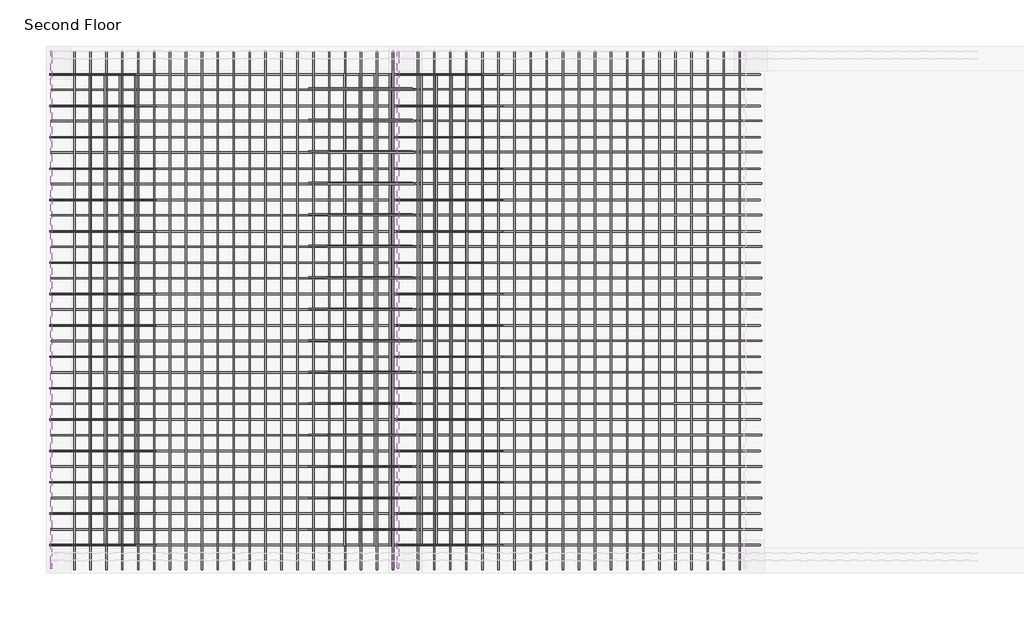
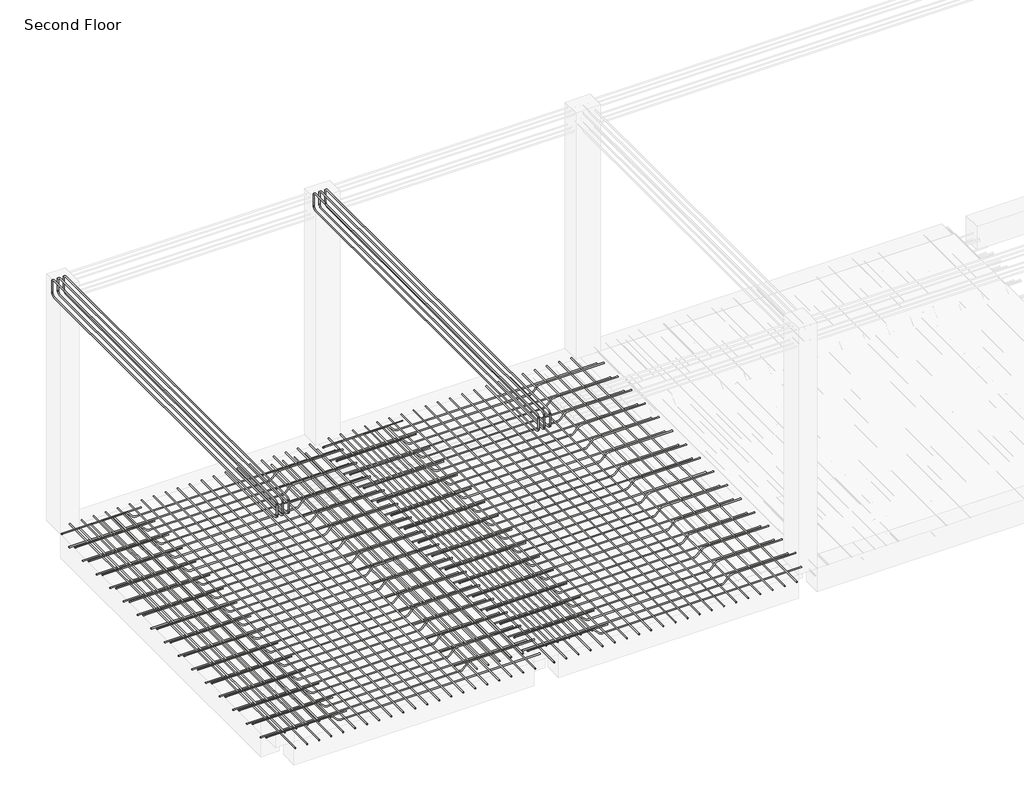
# One storey, part 2 of 4: 16 reinforcing bars.
"""IFC4 building model written with IfcOpenShell, lengths in millimetres."""

from ifc_helpers import new_model, si_unit, point, frame, origin, place, context, project, spatial, polyline, circle_curve, trimmed, segment, composite_curve, source, transform, mapped, element, save
from ifc_brep_helpers import swept_disk

model = new_model("IFC4")

# Units and contexts
model_context = context("Model", 3, world=origin())
ifc_project = project(units=[si_unit("LENGTHUNIT", "METRE", prefix="MILLI")], contexts=[model_context])

# Site, building, storey
site = spatial("IfcSite", under=ifc_project)
building = spatial("IfcBuilding", under=site)
storey = spatial("IfcBuildingStorey", under=building, Name="Second Floor", Elevation=6400.8)

# Reinforcing bars
placement = place(None, origin())
reinforcing_bar_shape = source(origin(), model_context, "Body", "SolidModel", [
    swept_disk(composite_curve([segment(polyline([(-6122.7112474, 5017.2334631, 9364.0994949), (-6122.7112474, 5017.2334631, 9512.0994949)]), True, "CONTINUOUS"), segment(trimmed(circle_curve(frame((-6122.7112474, 4971.2334631, 9512.0994949), z_axis=(1.0, 0.0, 0.0), x_axis=(0.0, 46.0, 0.0)), 46.0), [point((-6122.7112474, 5017.2334631, 9512.0994949))], [point((-6122.7112474, 4971.2334631, 9558.0994949))], True, "CARTESIAN"), True, "CONTINUOUS"), segment(polyline([(-6122.7112474, 4971.2334631, 9558.0994949), (-6122.7112474, 278.4334631, 9558.0994949)]), True, "CONTINUOUS"), segment(trimmed(circle_curve(frame((-6122.7112474, 278.4334631, 9512.0994949), z_axis=(1.0, 0.0, 0.0), x_axis=(0.0, 0.0, 46.0)), 46.0), [point((-6122.7112474, 278.4334631, 9558.0994949))], [point((-6122.7112474, 232.4334631, 9512.0994949))], True, "CARTESIAN"), True, "CONTINUOUS"), segment(polyline([(-6122.7112474, 232.4334631, 9512.0994949), (-6122.7112474, 232.4334631, 9364.0994949)]), True, "CONTINUOUS")], self_intersect=False), 6.0),
])
element("IfcReinforcingBar", 1, at=placement, inside=storey, context=model_context, shape_type="MappedRepresentation", body=[
    mapped(reinforcing_bar_shape, transform((0.0, 0.0, 0.0), x_axis=(1.0, 0.0, 0.0), y_axis=(0.0, 1.0, 0.0), z_axis=(0.0, 0.0, 1.0))),
    mapped(reinforcing_bar_shape, transform((71.1994949, 0.0, 0.0), x_axis=(1.0, 0.0, 0.0), y_axis=(0.0, 1.0, 0.0), z_axis=(0.0, 0.0, 1.0))),
    mapped(reinforcing_bar_shape, transform((142.3989899, 0.0, 0.0), x_axis=(1.0, 0.0, 0.0), y_axis=(0.0, 1.0, 0.0), z_axis=(0.0, 0.0, 1.0))),
])
reinforcing_bar_2_shape = source(origin(), model_context, "Body", "SolidModel", [
    swept_disk(composite_curve([segment(polyline([(-6122.7112474, 5017.2334631, 9533.5005051), (-6122.7112474, 5017.2334631, 9385.5005051)]), True, "CONTINUOUS"), segment(trimmed(circle_curve(frame((-6122.7112474, 4971.2334631, 9385.5005051), z_axis=(-1.0, 0.0, 0.0), x_axis=(0.0, 46.0, 0.0)), 46.0), [point((-6122.7112474, 5017.2334631, 9385.5005051))], [point((-6122.7112474, 4971.2334631, 9339.5005051))], True, "CARTESIAN"), True, "CONTINUOUS"), segment(polyline([(-6122.7112474, 4971.2334631, 9339.5005051), (-6122.7112474, 278.4334631, 9339.5005051)]), True, "CONTINUOUS"), segment(trimmed(circle_curve(frame((-6122.7112474, 278.4334631, 9385.5005051), z_axis=(-1.0, 0.0, 0.0), x_axis=(0.0, 0.0, -46.0)), 46.0), [point((-6122.7112474, 278.4334631, 9339.5005051))], [point((-6122.7112474, 232.4334631, 9385.5005051))], True, "CARTESIAN"), True, "CONTINUOUS"), segment(polyline([(-6122.7112474, 232.4334631, 9385.5005051), (-6122.7112474, 232.4334631, 9533.5005051)]), True, "CONTINUOUS")], self_intersect=False), 6.0),
])
element("IfcReinforcingBar", 2, at=placement, inside=storey, context=model_context, shape_type="MappedRepresentation", body=[
    mapped(reinforcing_bar_2_shape, transform((0.0, 0.0, 0.0), x_axis=(1.0, 0.0, 0.0), y_axis=(0.0, 1.0, 0.0), z_axis=(0.0, 0.0, 1.0))),
    mapped(reinforcing_bar_2_shape, transform((71.1994949, 0.0, 0.0), x_axis=(1.0, 0.0, 0.0), y_axis=(0.0, 1.0, 0.0), z_axis=(0.0, 0.0, 1.0))),
    mapped(reinforcing_bar_2_shape, transform((142.3989899, 0.0, 0.0), x_axis=(1.0, 0.0, 0.0), y_axis=(0.0, 1.0, 0.0), z_axis=(0.0, 0.0, 1.0))),
])
reinforcing_bar_3_shape = source(origin(), model_context, "Body", "SolidModel", [
    swept_disk(composite_curve([segment(polyline([(-9335.8112474, 5017.2334631, 9364.0994949), (-9335.8112474, 5017.2334631, 9512.0994949)]), True, "CONTINUOUS"), segment(trimmed(circle_curve(frame((-9335.8112474, 4971.2334631, 9512.0994949), z_axis=(1.0, 0.0, 0.0), x_axis=(0.0, 46.0, 0.0)), 46.0), [point((-9335.8112474, 5017.2334631, 9512.0994949))], [point((-9335.8112474, 4971.2334631, 9558.0994949))], True, "CARTESIAN"), True, "CONTINUOUS"), segment(polyline([(-9335.8112474, 4971.2334631, 9558.0994949), (-9335.8112474, 278.4334631, 9558.0994949)]), True, "CONTINUOUS"), segment(trimmed(circle_curve(frame((-9335.8112474, 278.4334631, 9512.0994949), z_axis=(1.0, 0.0, 0.0), x_axis=(0.0, 0.0, 46.0)), 46.0), [point((-9335.8112474, 278.4334631, 9558.0994949))], [point((-9335.8112474, 232.4334631, 9512.0994949))], True, "CARTESIAN"), True, "CONTINUOUS"), segment(polyline([(-9335.8112474, 232.4334631, 9512.0994949), (-9335.8112474, 232.4334631, 9364.0994949)]), True, "CONTINUOUS")], self_intersect=False), 6.0),
])
element("IfcReinforcingBar", 3, at=placement, inside=storey, context=model_context, shape_type="MappedRepresentation", body=[
    mapped(reinforcing_bar_3_shape, transform((0.0, 0.0, 0.0), x_axis=(1.0, 0.0, 0.0), y_axis=(0.0, 1.0, 0.0), z_axis=(0.0, 0.0, 1.0))),
    mapped(reinforcing_bar_3_shape, transform((71.1994949, 0.0, 0.0), x_axis=(1.0, 0.0, 0.0), y_axis=(0.0, 1.0, 0.0), z_axis=(0.0, 0.0, 1.0))),
    mapped(reinforcing_bar_3_shape, transform((142.3989899, 0.0, 0.0), x_axis=(1.0, 0.0, 0.0), y_axis=(0.0, 1.0, 0.0), z_axis=(0.0, 0.0, 1.0))),
])
reinforcing_bar_4_shape = source(origin(), model_context, "Body", "SolidModel", [
    swept_disk(composite_curve([segment(polyline([(-9335.8112474, 5017.2334631, 9533.5005051), (-9335.8112474, 5017.2334631, 9385.5005051)]), True, "CONTINUOUS"), segment(trimmed(circle_curve(frame((-9335.8112474, 4971.2334631, 9385.5005051), z_axis=(-1.0, 0.0, 0.0), x_axis=(0.0, 46.0, 0.0)), 46.0), [point((-9335.8112474, 5017.2334631, 9385.5005051))], [point((-9335.8112474, 4971.2334631, 9339.5005051))], True, "CARTESIAN"), True, "CONTINUOUS"), segment(polyline([(-9335.8112474, 4971.2334631, 9339.5005051), (-9335.8112474, 278.4334631, 9339.5005051)]), True, "CONTINUOUS"), segment(trimmed(circle_curve(frame((-9335.8112474, 278.4334631, 9385.5005051), z_axis=(-1.0, 0.0, 0.0), x_axis=(0.0, 0.0, -46.0)), 46.0), [point((-9335.8112474, 278.4334631, 9339.5005051))], [point((-9335.8112474, 232.4334631, 9385.5005051))], True, "CARTESIAN"), True, "CONTINUOUS"), segment(polyline([(-9335.8112474, 232.4334631, 9385.5005051), (-9335.8112474, 232.4334631, 9533.5005051)]), True, "CONTINUOUS")], self_intersect=False), 6.0),
])
element("IfcReinforcingBar", 4, at=placement, inside=storey, context=model_context, shape_type="MappedRepresentation", body=[
    mapped(reinforcing_bar_4_shape, transform((0.0, 0.0, 0.0), x_axis=(1.0, 0.0, 0.0), y_axis=(0.0, 1.0, 0.0), z_axis=(0.0, 0.0, 1.0))),
    mapped(reinforcing_bar_4_shape, transform((71.1994949, 0.0, 0.0), x_axis=(1.0, 0.0, 0.0), y_axis=(0.0, 1.0, 0.0), z_axis=(0.0, 0.0, 1.0))),
    mapped(reinforcing_bar_4_shape, transform((142.3989899, 0.0, 0.0), x_axis=(1.0, 0.0, 0.0), y_axis=(0.0, 1.0, 0.0), z_axis=(0.0, 0.0, 1.0))),
])
reinforcing_bar_5_shape = source(origin(), model_context, "Body", "SolidModel", [
    swept_disk(composite_curve([segment(polyline([(-9347.5125695, 4803.6334631, 6369.8), (-8565.5792829, 4803.6334631, 6369.8)]), True, "CONTINUOUS"), segment(trimmed(circle_curve(frame((-8565.5792829, 4803.6334631, 6323.8), z_axis=(0.0, 1.0, 0.0), x_axis=(0.0, 0.0, 46.0)), 46.0), [point((-8565.5792829, 4803.6334631, 6369.8))], [point((-8533.052371, 4803.6334631, 6356.3269119))], True, "CARTESIAN"), True, "CONTINUOUS"), segment(polyline([(-8533.052371, 4803.6334631, 6356.3269119), (-8469.5985471, 4803.6334631, 6292.8730881)]), True, "CONTINUOUS"), segment(trimmed(circle_curve(frame((-8437.0716352, 4803.6334631, 6325.4), z_axis=(0.0, -1.0000000000000002, 0.0), x_axis=(-32.526911900000414, 0.0, -32.526911899999504)), 46.0), [point((-8469.5985471, 4803.6334631, 6292.8730881))], [point((-8437.0716352, 4803.6334631, 6279.4))], True, "CARTESIAN"), True, "CONTINUOUS"), segment(polyline([(-8437.0716352, 4803.6334631, 6279.4), (-5982.0597449, 4803.6334631, 6279.4)]), True, "CONTINUOUS")], self_intersect=False), 6.0),
])
element("IfcReinforcingBar", 5, at=placement, inside=storey, context=model_context, shape_type="MappedRepresentation", body=[
    mapped(reinforcing_bar_5_shape, transform((0.0, 0.0, 0.0), x_axis=(1.0, 0.0, 0.0), y_axis=(0.0, 1.0, 0.0), z_axis=(0.0, 0.0, 1.0))),
    mapped(reinforcing_bar_5_shape, transform((0.0, -290.5066667, 0.0), x_axis=(1.0, 0.0, 0.0), y_axis=(0.0, 1.0, 0.0), z_axis=(0.0, 0.0, 1.0))),
    mapped(reinforcing_bar_5_shape, transform((0.0, -581.0133333, 0.0), x_axis=(1.0, 0.0, 0.0), y_axis=(0.0, 1.0, 0.0), z_axis=(0.0, 0.0, 1.0))),
    mapped(reinforcing_bar_5_shape, transform((0.0, -871.52, 0.0), x_axis=(1.0, 0.0, 0.0), y_axis=(0.0, 1.0, 0.0), z_axis=(0.0, 0.0, 1.0))),
    mapped(reinforcing_bar_5_shape, transform((0.0, -1162.0266667, 0.0), x_axis=(1.0, 0.0, 0.0), y_axis=(0.0, 1.0, 0.0), z_axis=(0.0, 0.0, 1.0))),
    mapped(reinforcing_bar_5_shape, transform((0.0, -1452.5333333, 0.0), x_axis=(1.0, 0.0, 0.0), y_axis=(0.0, 1.0, 0.0), z_axis=(0.0, 0.0, 1.0))),
    mapped(reinforcing_bar_5_shape, transform((0.0, -1743.04, 0.0), x_axis=(1.0, 0.0, 0.0), y_axis=(0.0, 1.0, 0.0), z_axis=(0.0, 0.0, 1.0))),
    mapped(reinforcing_bar_5_shape, transform((0.0, -2033.5466667, 0.0), x_axis=(1.0, 0.0, 0.0), y_axis=(0.0, 1.0, 0.0), z_axis=(0.0, 0.0, 1.0))),
    mapped(reinforcing_bar_5_shape, transform((0.0, -2324.0533333, 0.0), x_axis=(1.0, 0.0, 0.0), y_axis=(0.0, 1.0, 0.0), z_axis=(0.0, 0.0, 1.0))),
    mapped(reinforcing_bar_5_shape, transform((0.0, -2614.56, 0.0), x_axis=(1.0, 0.0, 0.0), y_axis=(0.0, 1.0, 0.0), z_axis=(0.0, 0.0, 1.0))),
    mapped(reinforcing_bar_5_shape, transform((0.0, -2905.0666667, 0.0), x_axis=(1.0, 0.0, 0.0), y_axis=(0.0, 1.0, 0.0), z_axis=(0.0, 0.0, 1.0))),
    mapped(reinforcing_bar_5_shape, transform((0.0, -3195.5733333, 0.0), x_axis=(1.0, 0.0, 0.0), y_axis=(0.0, 1.0, 0.0), z_axis=(0.0, 0.0, 1.0))),
    mapped(reinforcing_bar_5_shape, transform((0.0, -3486.08, 0.0), x_axis=(1.0, 0.0, 0.0), y_axis=(0.0, 1.0, 0.0), z_axis=(0.0, 0.0, 1.0))),
    mapped(reinforcing_bar_5_shape, transform((0.0, -3776.5866667, 0.0), x_axis=(1.0, 0.0, 0.0), y_axis=(0.0, 1.0, 0.0), z_axis=(0.0, 0.0, 1.0))),
    mapped(reinforcing_bar_5_shape, transform((0.0, -4067.0933333, 0.0), x_axis=(1.0, 0.0, 0.0), y_axis=(0.0, 1.0, 0.0), z_axis=(0.0, 0.0, 1.0))),
    mapped(reinforcing_bar_5_shape, transform((0.0, -4357.6, 0.0), x_axis=(1.0, 0.0, 0.0), y_axis=(0.0, 1.0, 0.0), z_axis=(0.0, 0.0, 1.0))),
])
reinforcing_bar_6_shape = source(origin(), model_context, "Body", "SolidModel", [
    swept_disk(composite_curve([segment(polyline([(-5968.6109354, 590.4513536, 6369.8), (-6750.544222, 590.4513536, 6369.8)]), True, "CONTINUOUS"), segment(trimmed(circle_curve(frame((-6750.544222, 590.4513536, 6323.8), z_axis=(0.0, -1.0, 0.0), x_axis=(0.0, 0.0, 46.0)), 46.0), [point((-6750.544222, 590.4513536, 6369.8))], [point((-6783.0711339, 590.4513536, 6356.3269119))], True, "CARTESIAN"), True, "CONTINUOUS"), segment(polyline([(-6783.0711339, 590.4513536, 6356.3269119), (-6846.5249578, 590.4513536, 6292.8730881)]), True, "CONTINUOUS"), segment(trimmed(circle_curve(frame((-6879.0518697, 590.4513536, 6325.4), z_axis=(0.0, 1.0000000000000002, 0.0), x_axis=(32.526911899999504, 0.0, -32.526911899999504)), 46.0), [point((-6846.5249578, 590.4513536, 6292.8730881))], [point((-6879.0518697, 590.4513536, 6279.4))], True, "CARTESIAN"), True, "CONTINUOUS"), segment(polyline([(-6879.0518697, 590.4513536, 6279.4), (-9334.06376, 590.4513536, 6279.4)]), True, "CONTINUOUS")], self_intersect=False), 6.0),
])
element("IfcReinforcingBar", 6, at=placement, inside=storey, context=model_context, shape_type="MappedRepresentation", body=[
    mapped(reinforcing_bar_6_shape, transform((0.0, 0.0, 0.0), x_axis=(1.0, 0.0, 0.0), y_axis=(0.0, 1.0, 0.0), z_axis=(0.0, 0.0, 1.0))),
    mapped(reinforcing_bar_6_shape, transform((0.0, 290.9296088, 0.0), x_axis=(1.0, 0.0, 0.0), y_axis=(0.0, 1.0, 0.0), z_axis=(0.0, 0.0, 1.0))),
    mapped(reinforcing_bar_6_shape, transform((0.0, 581.8592177, 0.0), x_axis=(1.0, 0.0, 0.0), y_axis=(0.0, 1.0, 0.0), z_axis=(0.0, 0.0, 1.0))),
    mapped(reinforcing_bar_6_shape, transform((0.0, 872.7888265, 0.0), x_axis=(1.0, 0.0, 0.0), y_axis=(0.0, 1.0, 0.0), z_axis=(0.0, 0.0, 1.0))),
    mapped(reinforcing_bar_6_shape, transform((0.0, 1163.7184353, 0.0), x_axis=(1.0, 0.0, 0.0), y_axis=(0.0, 1.0, 0.0), z_axis=(0.0, 0.0, 1.0))),
    mapped(reinforcing_bar_6_shape, transform((0.0, 1454.6480442, 0.0), x_axis=(1.0, 0.0, 0.0), y_axis=(0.0, 1.0, 0.0), z_axis=(0.0, 0.0, 1.0))),
    mapped(reinforcing_bar_6_shape, transform((0.0, 1745.577653, 0.0), x_axis=(1.0, 0.0, 0.0), y_axis=(0.0, 1.0, 0.0), z_axis=(0.0, 0.0, 1.0))),
    mapped(reinforcing_bar_6_shape, transform((0.0, 2036.5072618, 0.0), x_axis=(1.0, 0.0, 0.0), y_axis=(0.0, 1.0, 0.0), z_axis=(0.0, 0.0, 1.0))),
    mapped(reinforcing_bar_6_shape, transform((0.0, 2327.4368707, 0.0), x_axis=(1.0, 0.0, 0.0), y_axis=(0.0, 1.0, 0.0), z_axis=(0.0, 0.0, 1.0))),
    mapped(reinforcing_bar_6_shape, transform((0.0, 2618.3664795, 0.0), x_axis=(1.0, 0.0, 0.0), y_axis=(0.0, 1.0, 0.0), z_axis=(0.0, 0.0, 1.0))),
    mapped(reinforcing_bar_6_shape, transform((0.0, 2909.2960883, 0.0), x_axis=(1.0, 0.0, 0.0), y_axis=(0.0, 1.0, 0.0), z_axis=(0.0, 0.0, 1.0))),
    mapped(reinforcing_bar_6_shape, transform((0.0, 3200.2256972, 0.0), x_axis=(1.0, 0.0, 0.0), y_axis=(0.0, 1.0, 0.0), z_axis=(0.0, 0.0, 1.0))),
    mapped(reinforcing_bar_6_shape, transform((0.0, 3491.155306, 0.0), x_axis=(1.0, 0.0, 0.0), y_axis=(0.0, 1.0, 0.0), z_axis=(0.0, 0.0, 1.0))),
    mapped(reinforcing_bar_6_shape, transform((0.0, 3782.0849148, 0.0), x_axis=(1.0, 0.0, 0.0), y_axis=(0.0, 1.0, 0.0), z_axis=(0.0, 0.0, 1.0))),
    mapped(reinforcing_bar_6_shape, transform((0.0, 4073.0145236, 0.0), x_axis=(1.0, 0.0, 0.0), y_axis=(0.0, 1.0, 0.0), z_axis=(0.0, 0.0, 1.0))),
])
reinforcing_bar_7_shape = source(origin(), model_context, "Body", "SolidModel", [
    swept_disk(composite_curve([segment(polyline([(-8556.5984173, 4809.6334631, 6359.5006995), (-8556.5984173, 440.0334631, 6359.5006995)]), True, "CONTINUOUS")], self_intersect=False), 6.0),
])
element("IfcReinforcingBar", 7, at=placement, inside=storey, context=model_context, shape_type="MappedRepresentation", body=[
    mapped(reinforcing_bar_7_shape, transform((0.0, 0.0, 0.0), x_axis=(1.0, 0.0, 0.0), y_axis=(0.0, 1.0, 0.0), z_axis=(0.0, 0.0, 1.0))),
    mapped(reinforcing_bar_7_shape, transform((-140.6783338, 0.0, 0.0), x_axis=(1.0, 0.0, 0.0), y_axis=(0.0, 1.0, 0.0), z_axis=(0.0, 0.0, 1.0))),
    mapped(reinforcing_bar_7_shape, transform((-281.3566676, 0.0, 0.0), x_axis=(1.0, 0.0, 0.0), y_axis=(0.0, 1.0, 0.0), z_axis=(0.0, 0.0, 1.0))),
    mapped(reinforcing_bar_7_shape, transform((-422.0350014, 0.0, 0.0), x_axis=(1.0, 0.0, 0.0), y_axis=(0.0, 1.0, 0.0), z_axis=(0.0, 0.0, 1.0))),
    mapped(reinforcing_bar_7_shape, transform((-562.7133352, 0.0, 0.0), x_axis=(1.0, 0.0, 0.0), y_axis=(0.0, 1.0, 0.0), z_axis=(0.0, 0.0, 1.0))),
])
reinforcing_bar_8_shape = source(origin(), model_context, "Body", "SolidModel", [
    swept_disk(composite_curve([segment(polyline([(-6759.5250876, 4809.6334631, 6359.5006995), (-6759.5250876, 440.0334631, 6359.5006995)]), True, "CONTINUOUS")], self_intersect=False), 6.0),
])
element("IfcReinforcingBar", 8, at=placement, inside=storey, context=model_context, shape_type="MappedRepresentation", body=[
    mapped(reinforcing_bar_8_shape, transform((0.0, 0.0, 0.0), x_axis=(1.0, 0.0, 0.0), y_axis=(0.0, 1.0, 0.0), z_axis=(0.0, 0.0, 1.0))),
    mapped(reinforcing_bar_8_shape, transform((140.6783338, 0.0, 0.0), x_axis=(1.0, 0.0, 0.0), y_axis=(0.0, 1.0, 0.0), z_axis=(0.0, 0.0, 1.0))),
    mapped(reinforcing_bar_8_shape, transform((281.3566676, 0.0, 0.0), x_axis=(1.0, 0.0, 0.0), y_axis=(0.0, 1.0, 0.0), z_axis=(0.0, 0.0, 1.0))),
    mapped(reinforcing_bar_8_shape, transform((422.0350014, 0.0, 0.0), x_axis=(1.0, 0.0, 0.0), y_axis=(0.0, 1.0, 0.0), z_axis=(0.0, 0.0, 1.0))),
    mapped(reinforcing_bar_8_shape, transform((562.7133352, 0.0, 0.0), x_axis=(1.0, 0.0, 0.0), y_axis=(0.0, 1.0, 0.0), z_axis=(0.0, 0.0, 1.0))),
])
reinforcing_bar_9_shape = source(origin(), model_context, "Body", "SolidModel", [
    swept_disk(composite_curve([segment(polyline([(-9338.4522926, 4805.6334631, 6371.8), (-8365.7369752, 4805.6334631, 6371.8)]), True, "CONTINUOUS")], self_intersect=False), 4.0),
])
element("IfcReinforcingBar", 9, at=placement, inside=storey, context=model_context, shape_type="MappedRepresentation", body=[
    mapped(reinforcing_bar_9_shape, transform((0.0, 0.0, 0.0), x_axis=(1.0, 0.0, 0.0), y_axis=(0.0, 1.0, 0.0), z_axis=(0.0, 0.0, 1.0))),
    mapped(reinforcing_bar_9_shape, transform((0.0, -290.7733333, 0.0), x_axis=(1.0, 0.0, 0.0), y_axis=(0.0, 1.0, 0.0), z_axis=(0.0, 0.0, 1.0))),
    mapped(reinforcing_bar_9_shape, transform((0.0, -581.5466667, 0.0), x_axis=(1.0, 0.0, 0.0), y_axis=(0.0, 1.0, 0.0), z_axis=(0.0, 0.0, 1.0))),
    mapped(reinforcing_bar_9_shape, transform((0.0, -872.32, 0.0), x_axis=(1.0, 0.0, 0.0), y_axis=(0.0, 1.0, 0.0), z_axis=(0.0, 0.0, 1.0))),
    mapped(reinforcing_bar_9_shape, transform((0.0, -1163.0933333, 0.0), x_axis=(1.0, 0.0, 0.0), y_axis=(0.0, 1.0, 0.0), z_axis=(0.0, 0.0, 1.0))),
    mapped(reinforcing_bar_9_shape, transform((0.0, -1453.8666667, 0.0), x_axis=(1.0, 0.0, 0.0), y_axis=(0.0, 1.0, 0.0), z_axis=(0.0, 0.0, 1.0))),
    mapped(reinforcing_bar_9_shape, transform((0.0, -1744.64, 0.0), x_axis=(1.0, 0.0, 0.0), y_axis=(0.0, 1.0, 0.0), z_axis=(0.0, 0.0, 1.0))),
    mapped(reinforcing_bar_9_shape, transform((0.0, -2035.4133333, 0.0), x_axis=(1.0, 0.0, 0.0), y_axis=(0.0, 1.0, 0.0), z_axis=(0.0, 0.0, 1.0))),
    mapped(reinforcing_bar_9_shape, transform((0.0, -2326.1866667, 0.0), x_axis=(1.0, 0.0, 0.0), y_axis=(0.0, 1.0, 0.0), z_axis=(0.0, 0.0, 1.0))),
    mapped(reinforcing_bar_9_shape, transform((0.0, -2616.96, 0.0), x_axis=(1.0, 0.0, 0.0), y_axis=(0.0, 1.0, 0.0), z_axis=(0.0, 0.0, 1.0))),
    mapped(reinforcing_bar_9_shape, transform((0.0, -2907.7333333, 0.0), x_axis=(1.0, 0.0, 0.0), y_axis=(0.0, 1.0, 0.0), z_axis=(0.0, 0.0, 1.0))),
    mapped(reinforcing_bar_9_shape, transform((0.0, -3198.5066667, 0.0), x_axis=(1.0, 0.0, 0.0), y_axis=(0.0, 1.0, 0.0), z_axis=(0.0, 0.0, 1.0))),
    mapped(reinforcing_bar_9_shape, transform((0.0, -3489.28, 0.0), x_axis=(1.0, 0.0, 0.0), y_axis=(0.0, 1.0, 0.0), z_axis=(0.0, 0.0, 1.0))),
    mapped(reinforcing_bar_9_shape, transform((0.0, -3780.0533333, 0.0), x_axis=(1.0, 0.0, 0.0), y_axis=(0.0, 1.0, 0.0), z_axis=(0.0, 0.0, 1.0))),
    mapped(reinforcing_bar_9_shape, transform((0.0, -4070.8266667, 0.0), x_axis=(1.0, 0.0, 0.0), y_axis=(0.0, 1.0, 0.0), z_axis=(0.0, 0.0, 1.0))),
    mapped(reinforcing_bar_9_shape, transform((0.0, -4361.6, 0.0), x_axis=(1.0, 0.0, 0.0), y_axis=(0.0, 1.0, 0.0), z_axis=(0.0, 0.0, 1.0))),
])
reinforcing_bar_10_shape = source(origin(), model_context, "Body", "SolidModel", [
    swept_disk(composite_curve([segment(polyline([(-5991.3123639, 4678.4115375, 6371.8), (-6950.3865297, 4678.4115375, 6371.8)]), True, "CONTINUOUS")], self_intersect=False), 4.0),
])
element("IfcReinforcingBar", 10, at=placement, inside=storey, context=model_context, shape_type="MappedRepresentation", body=[
    mapped(reinforcing_bar_10_shape, transform((0.0, 0.0, 0.0), x_axis=(1.0, 0.0, 0.0), y_axis=(0.0, 1.0, 0.0), z_axis=(0.0, 0.0, 1.0))),
    mapped(reinforcing_bar_10_shape, transform((0.0, -291.8025106, 0.0), x_axis=(1.0, 0.0, 0.0), y_axis=(0.0, 1.0, 0.0), z_axis=(0.0, 0.0, 1.0))),
    mapped(reinforcing_bar_10_shape, transform((0.0, -583.6050212, 0.0), x_axis=(1.0, 0.0, 0.0), y_axis=(0.0, 1.0, 0.0), z_axis=(0.0, 0.0, 1.0))),
    mapped(reinforcing_bar_10_shape, transform((0.0, -875.4075319, 0.0), x_axis=(1.0, 0.0, 0.0), y_axis=(0.0, 1.0, 0.0), z_axis=(0.0, 0.0, 1.0))),
    mapped(reinforcing_bar_10_shape, transform((0.0, -1167.2100425, 0.0), x_axis=(1.0, 0.0, 0.0), y_axis=(0.0, 1.0, 0.0), z_axis=(0.0, 0.0, 1.0))),
    mapped(reinforcing_bar_10_shape, transform((0.0, -1459.0125531, 0.0), x_axis=(1.0, 0.0, 0.0), y_axis=(0.0, 1.0, 0.0), z_axis=(0.0, 0.0, 1.0))),
    mapped(reinforcing_bar_10_shape, transform((0.0, -1750.8150637, 0.0), x_axis=(1.0, 0.0, 0.0), y_axis=(0.0, 1.0, 0.0), z_axis=(0.0, 0.0, 1.0))),
    mapped(reinforcing_bar_10_shape, transform((0.0, -2042.6175743, 0.0), x_axis=(1.0, 0.0, 0.0), y_axis=(0.0, 1.0, 0.0), z_axis=(0.0, 0.0, 1.0))),
    mapped(reinforcing_bar_10_shape, transform((0.0, -2334.420085, 0.0), x_axis=(1.0, 0.0, 0.0), y_axis=(0.0, 1.0, 0.0), z_axis=(0.0, 0.0, 1.0))),
    mapped(reinforcing_bar_10_shape, transform((0.0, -2626.2225956, 0.0), x_axis=(1.0, 0.0, 0.0), y_axis=(0.0, 1.0, 0.0), z_axis=(0.0, 0.0, 1.0))),
    mapped(reinforcing_bar_10_shape, transform((0.0, -2918.0251062, 0.0), x_axis=(1.0, 0.0, 0.0), y_axis=(0.0, 1.0, 0.0), z_axis=(0.0, 0.0, 1.0))),
    mapped(reinforcing_bar_10_shape, transform((0.0, -3209.8276168, 0.0), x_axis=(1.0, 0.0, 0.0), y_axis=(0.0, 1.0, 0.0), z_axis=(0.0, 0.0, 1.0))),
    mapped(reinforcing_bar_10_shape, transform((0.0, -3501.6301274, 0.0), x_axis=(1.0, 0.0, 0.0), y_axis=(0.0, 1.0, 0.0), z_axis=(0.0, 0.0, 1.0))),
    mapped(reinforcing_bar_10_shape, transform((0.0, -3793.4326381, 0.0), x_axis=(1.0, 0.0, 0.0), y_axis=(0.0, 1.0, 0.0), z_axis=(0.0, 0.0, 1.0))),
    mapped(reinforcing_bar_10_shape, transform((0.0, -4085.2351487, 0.0), x_axis=(1.0, 0.0, 0.0), y_axis=(0.0, 1.0, 0.0), z_axis=(0.0, 0.0, 1.0))),
])
reinforcing_bar_11_shape = source(origin(), model_context, "Body", "SolidModel", [
    swept_disk(composite_curve([segment(polyline([(-6169.8117524, 218.9117605, 6287.9387401), (-6169.8117524, 5019.9992064, 6287.9387401)]), True, "CONTINUOUS")], self_intersect=False), 6.0),
])
element("IfcReinforcingBar", 11, at=placement, inside=storey, context=model_context, shape_type="MappedRepresentation", body=[
    mapped(reinforcing_bar_11_shape, transform((0.0, 0.0, 0.0), x_axis=(1.0, 0.0, 0.0), y_axis=(0.0, 1.0, 0.0), z_axis=(0.0, 0.0, 1.0))),
    mapped(reinforcing_bar_11_shape, transform((-147.475, 0.0, 0.0), x_axis=(1.0, 0.0, 0.0), y_axis=(0.0, 1.0, 0.0), z_axis=(0.0, 0.0, 1.0))),
    mapped(reinforcing_bar_11_shape, transform((-294.95, 0.0, 0.0), x_axis=(1.0, 0.0, 0.0), y_axis=(0.0, 1.0, 0.0), z_axis=(0.0, 0.0, 1.0))),
    mapped(reinforcing_bar_11_shape, transform((-442.425, 0.0, 0.0), x_axis=(1.0, 0.0, 0.0), y_axis=(0.0, 1.0, 0.0), z_axis=(0.0, 0.0, 1.0))),
    mapped(reinforcing_bar_11_shape, transform((-589.9, 0.0, 0.0), x_axis=(1.0, 0.0, 0.0), y_axis=(0.0, 1.0, 0.0), z_axis=(0.0, 0.0, 1.0))),
    mapped(reinforcing_bar_11_shape, transform((-737.375, 0.0, 0.0), x_axis=(1.0, 0.0, 0.0), y_axis=(0.0, 1.0, 0.0), z_axis=(0.0, 0.0, 1.0))),
    mapped(reinforcing_bar_11_shape, transform((-884.85, 0.0, 0.0), x_axis=(1.0, 0.0, 0.0), y_axis=(0.0, 1.0, 0.0), z_axis=(0.0, 0.0, 1.0))),
    mapped(reinforcing_bar_11_shape, transform((-1032.325, 0.0, 0.0), x_axis=(1.0, 0.0, 0.0), y_axis=(0.0, 1.0, 0.0), z_axis=(0.0, 0.0, 1.0))),
    mapped(reinforcing_bar_11_shape, transform((-1179.8, 0.0, 0.0), x_axis=(1.0, 0.0, 0.0), y_axis=(0.0, 1.0, 0.0), z_axis=(0.0, 0.0, 1.0))),
    mapped(reinforcing_bar_11_shape, transform((-1327.275, 0.0, 0.0), x_axis=(1.0, 0.0, 0.0), y_axis=(0.0, 1.0, 0.0), z_axis=(0.0, 0.0, 1.0))),
    mapped(reinforcing_bar_11_shape, transform((-1474.75, 0.0, 0.0), x_axis=(1.0, 0.0, 0.0), y_axis=(0.0, 1.0, 0.0), z_axis=(0.0, 0.0, 1.0))),
    mapped(reinforcing_bar_11_shape, transform((-1622.225, 0.0, 0.0), x_axis=(1.0, 0.0, 0.0), y_axis=(0.0, 1.0, 0.0), z_axis=(0.0, 0.0, 1.0))),
    mapped(reinforcing_bar_11_shape, transform((-1769.7, 0.0, 0.0), x_axis=(1.0, 0.0, 0.0), y_axis=(0.0, 1.0, 0.0), z_axis=(0.0, 0.0, 1.0))),
    mapped(reinforcing_bar_11_shape, transform((-1917.175, 0.0, 0.0), x_axis=(1.0, 0.0, 0.0), y_axis=(0.0, 1.0, 0.0), z_axis=(0.0, 0.0, 1.0))),
    mapped(reinforcing_bar_11_shape, transform((-2064.65, 0.0, 0.0), x_axis=(1.0, 0.0, 0.0), y_axis=(0.0, 1.0, 0.0), z_axis=(0.0, 0.0, 1.0))),
    mapped(reinforcing_bar_11_shape, transform((-2212.125, 0.0, 0.0), x_axis=(1.0, 0.0, 0.0), y_axis=(0.0, 1.0, 0.0), z_axis=(0.0, 0.0, 1.0))),
    mapped(reinforcing_bar_11_shape, transform((-2359.6, 0.0, 0.0), x_axis=(1.0, 0.0, 0.0), y_axis=(0.0, 1.0, 0.0), z_axis=(0.0, 0.0, 1.0))),
    mapped(reinforcing_bar_11_shape, transform((-2507.075, 0.0, 0.0), x_axis=(1.0, 0.0, 0.0), y_axis=(0.0, 1.0, 0.0), z_axis=(0.0, 0.0, 1.0))),
    mapped(reinforcing_bar_11_shape, transform((-2654.55, 0.0, 0.0), x_axis=(1.0, 0.0, 0.0), y_axis=(0.0, 1.0, 0.0), z_axis=(0.0, 0.0, 1.0))),
    mapped(reinforcing_bar_11_shape, transform((-2802.025, 0.0, 0.0), x_axis=(1.0, 0.0, 0.0), y_axis=(0.0, 1.0, 0.0), z_axis=(0.0, 0.0, 1.0))),
    mapped(reinforcing_bar_11_shape, transform((-2949.5, 0.0, 0.0), x_axis=(1.0, 0.0, 0.0), y_axis=(0.0, 1.0, 0.0), z_axis=(0.0, 0.0, 1.0))),
])
reinforcing_bar_12_shape = source(origin(), model_context, "Body", "SolidModel", [
    swept_disk(composite_curve([segment(polyline([(-6134.4125695, 4803.6334631, 6369.8), (-5352.4792829, 4803.6334631, 6369.8)]), True, "CONTINUOUS"), segment(trimmed(circle_curve(frame((-5352.4792829, 4803.6334631, 6323.8), z_axis=(0.0, 1.0, 0.0), x_axis=(0.0, 0.0, 46.0)), 46.0), [point((-5352.4792829, 4803.6334631, 6369.8))], [point((-5319.952371, 4803.6334631, 6356.3269119))], True, "CARTESIAN"), True, "CONTINUOUS"), segment(polyline([(-5319.952371, 4803.6334631, 6356.3269119), (-5256.4985471, 4803.6334631, 6292.8730881)]), True, "CONTINUOUS"), segment(trimmed(circle_curve(frame((-5223.9716352, 4803.6334631, 6325.4), z_axis=(0.0, -1.0000000000000002, 0.0), x_axis=(-32.526911900000414, 0.0, -32.526911899999504)), 46.0), [point((-5256.4985471, 4803.6334631, 6292.8730881))], [point((-5223.9716352, 4803.6334631, 6279.4))], True, "CARTESIAN"), True, "CONTINUOUS"), segment(polyline([(-5223.9716352, 4803.6334631, 6279.4), (-2768.9597449, 4803.6334631, 6279.4)]), True, "CONTINUOUS")], self_intersect=False), 6.0),
])
element("IfcReinforcingBar", 12, at=placement, inside=storey, context=model_context, shape_type="MappedRepresentation", body=[
    mapped(reinforcing_bar_12_shape, transform((0.0, 0.0, 0.0), x_axis=(1.0, 0.0, 0.0), y_axis=(0.0, 1.0, 0.0), z_axis=(0.0, 0.0, 1.0))),
    mapped(reinforcing_bar_12_shape, transform((0.0, -290.5066667, 0.0), x_axis=(1.0, 0.0, 0.0), y_axis=(0.0, 1.0, 0.0), z_axis=(0.0, 0.0, 1.0))),
    mapped(reinforcing_bar_12_shape, transform((0.0, -581.0133333, 0.0), x_axis=(1.0, 0.0, 0.0), y_axis=(0.0, 1.0, 0.0), z_axis=(0.0, 0.0, 1.0))),
    mapped(reinforcing_bar_12_shape, transform((0.0, -871.52, 0.0), x_axis=(1.0, 0.0, 0.0), y_axis=(0.0, 1.0, 0.0), z_axis=(0.0, 0.0, 1.0))),
    mapped(reinforcing_bar_12_shape, transform((0.0, -1162.0266667, 0.0), x_axis=(1.0, 0.0, 0.0), y_axis=(0.0, 1.0, 0.0), z_axis=(0.0, 0.0, 1.0))),
    mapped(reinforcing_bar_12_shape, transform((0.0, -1452.5333333, 0.0), x_axis=(1.0, 0.0, 0.0), y_axis=(0.0, 1.0, 0.0), z_axis=(0.0, 0.0, 1.0))),
    mapped(reinforcing_bar_12_shape, transform((0.0, -1743.04, 0.0), x_axis=(1.0, 0.0, 0.0), y_axis=(0.0, 1.0, 0.0), z_axis=(0.0, 0.0, 1.0))),
    mapped(reinforcing_bar_12_shape, transform((0.0, -2033.5466667, 0.0), x_axis=(1.0, 0.0, 0.0), y_axis=(0.0, 1.0, 0.0), z_axis=(0.0, 0.0, 1.0))),
    mapped(reinforcing_bar_12_shape, transform((0.0, -2324.0533333, 0.0), x_axis=(1.0, 0.0, 0.0), y_axis=(0.0, 1.0, 0.0), z_axis=(0.0, 0.0, 1.0))),
    mapped(reinforcing_bar_12_shape, transform((0.0, -2614.56, 0.0), x_axis=(1.0, 0.0, 0.0), y_axis=(0.0, 1.0, 0.0), z_axis=(0.0, 0.0, 1.0))),
    mapped(reinforcing_bar_12_shape, transform((0.0, -2905.0666667, 0.0), x_axis=(1.0, 0.0, 0.0), y_axis=(0.0, 1.0, 0.0), z_axis=(0.0, 0.0, 1.0))),
    mapped(reinforcing_bar_12_shape, transform((0.0, -3195.5733333, 0.0), x_axis=(1.0, 0.0, 0.0), y_axis=(0.0, 1.0, 0.0), z_axis=(0.0, 0.0, 1.0))),
    mapped(reinforcing_bar_12_shape, transform((0.0, -3486.08, 0.0), x_axis=(1.0, 0.0, 0.0), y_axis=(0.0, 1.0, 0.0), z_axis=(0.0, 0.0, 1.0))),
    mapped(reinforcing_bar_12_shape, transform((0.0, -3776.5866667, 0.0), x_axis=(1.0, 0.0, 0.0), y_axis=(0.0, 1.0, 0.0), z_axis=(0.0, 0.0, 1.0))),
    mapped(reinforcing_bar_12_shape, transform((0.0, -4067.0933333, 0.0), x_axis=(1.0, 0.0, 0.0), y_axis=(0.0, 1.0, 0.0), z_axis=(0.0, 0.0, 1.0))),
    mapped(reinforcing_bar_12_shape, transform((0.0, -4357.6, 0.0), x_axis=(1.0, 0.0, 0.0), y_axis=(0.0, 1.0, 0.0), z_axis=(0.0, 0.0, 1.0))),
])
reinforcing_bar_13_shape = source(origin(), model_context, "Body", "SolidModel", [
    swept_disk(composite_curve([segment(polyline([(-2755.5109354, 590.4513536, 6369.8), (-3537.444222, 590.4513536, 6369.8)]), True, "CONTINUOUS"), segment(trimmed(circle_curve(frame((-3537.444222, 590.4513536, 6323.8), z_axis=(0.0, -1.0, 0.0), x_axis=(0.0, 0.0, 46.0)), 46.0), [point((-3537.444222, 590.4513536, 6369.8))], [point((-3569.9711339, 590.4513536, 6356.3269119))], True, "CARTESIAN"), True, "CONTINUOUS"), segment(polyline([(-3569.9711339, 590.4513536, 6356.3269119), (-3633.4249578, 590.4513536, 6292.8730881)]), True, "CONTINUOUS"), segment(trimmed(circle_curve(frame((-3665.9518697, 590.4513536, 6325.4), z_axis=(0.0, 1.0000000000000002, 0.0), x_axis=(32.52691189999996, 0.0, -32.526911899999504)), 46.0), [point((-3633.4249578, 590.4513536, 6292.8730881))], [point((-3665.9518697, 590.4513536, 6279.4))], True, "CARTESIAN"), True, "CONTINUOUS"), segment(polyline([(-3665.9518697, 590.4513536, 6279.4), (-6120.96376, 590.4513536, 6279.4)]), True, "CONTINUOUS")], self_intersect=False), 6.0),
])
element("IfcReinforcingBar", 13, at=placement, inside=storey, context=model_context, shape_type="MappedRepresentation", body=[
    mapped(reinforcing_bar_13_shape, transform((0.0, 0.0, 0.0), x_axis=(1.0, 0.0, 0.0), y_axis=(0.0, 1.0, 0.0), z_axis=(0.0, 0.0, 1.0))),
    mapped(reinforcing_bar_13_shape, transform((0.0, 291.2629007, 0.0), x_axis=(1.0, 0.0, 0.0), y_axis=(0.0, 1.0, 0.0), z_axis=(0.0, 0.0, 1.0))),
    mapped(reinforcing_bar_13_shape, transform((0.0, 582.5258014, 0.0), x_axis=(1.0, 0.0, 0.0), y_axis=(0.0, 1.0, 0.0), z_axis=(0.0, 0.0, 1.0))),
    mapped(reinforcing_bar_13_shape, transform((0.0, 873.7887021, 0.0), x_axis=(1.0, 0.0, 0.0), y_axis=(0.0, 1.0, 0.0), z_axis=(0.0, 0.0, 1.0))),
    mapped(reinforcing_bar_13_shape, transform((0.0, 1165.0516028, 0.0), x_axis=(1.0, 0.0, 0.0), y_axis=(0.0, 1.0, 0.0), z_axis=(0.0, 0.0, 1.0))),
    mapped(reinforcing_bar_13_shape, transform((0.0, 1456.3145035, 0.0), x_axis=(1.0, 0.0, 0.0), y_axis=(0.0, 1.0, 0.0), z_axis=(0.0, 0.0, 1.0))),
    mapped(reinforcing_bar_13_shape, transform((0.0, 1747.5774042, 0.0), x_axis=(1.0, 0.0, 0.0), y_axis=(0.0, 1.0, 0.0), z_axis=(0.0, 0.0, 1.0))),
    mapped(reinforcing_bar_13_shape, transform((0.0, 2038.8403049, 0.0), x_axis=(1.0, 0.0, 0.0), y_axis=(0.0, 1.0, 0.0), z_axis=(0.0, 0.0, 1.0))),
    mapped(reinforcing_bar_13_shape, transform((0.0, 2330.1032056, 0.0), x_axis=(1.0, 0.0, 0.0), y_axis=(0.0, 1.0, 0.0), z_axis=(0.0, 0.0, 1.0))),
    mapped(reinforcing_bar_13_shape, transform((0.0, 2621.3661063, 0.0), x_axis=(1.0, 0.0, 0.0), y_axis=(0.0, 1.0, 0.0), z_axis=(0.0, 0.0, 1.0))),
    mapped(reinforcing_bar_13_shape, transform((0.0, 2912.629007, 0.0), x_axis=(1.0, 0.0, 0.0), y_axis=(0.0, 1.0, 0.0), z_axis=(0.0, 0.0, 1.0))),
    mapped(reinforcing_bar_13_shape, transform((0.0, 3203.8919077, 0.0), x_axis=(1.0, 0.0, 0.0), y_axis=(0.0, 1.0, 0.0), z_axis=(0.0, 0.0, 1.0))),
    mapped(reinforcing_bar_13_shape, transform((0.0, 3495.1548084, 0.0), x_axis=(1.0, 0.0, 0.0), y_axis=(0.0, 1.0, 0.0), z_axis=(0.0, 0.0, 1.0))),
    mapped(reinforcing_bar_13_shape, transform((0.0, 3786.4177091, 0.0), x_axis=(1.0, 0.0, 0.0), y_axis=(0.0, 1.0, 0.0), z_axis=(0.0, 0.0, 1.0))),
    mapped(reinforcing_bar_13_shape, transform((0.0, 4077.6806098, 0.0), x_axis=(1.0, 0.0, 0.0), y_axis=(0.0, 1.0, 0.0), z_axis=(0.0, 0.0, 1.0))),
])
reinforcing_bar_14_shape = source(origin(), model_context, "Body", "SolidModel", [
    swept_disk(composite_curve([segment(polyline([(-6125.3522926, 4805.6334631, 6371.8), (-5152.6369752, 4805.6334631, 6371.8)]), True, "CONTINUOUS")], self_intersect=False), 4.0),
])
element("IfcReinforcingBar", 14, at=placement, inside=storey, context=model_context, shape_type="MappedRepresentation", body=[
    mapped(reinforcing_bar_14_shape, transform((0.0, 0.0, 0.0), x_axis=(1.0, 0.0, 0.0), y_axis=(0.0, 1.0, 0.0), z_axis=(0.0, 0.0, 1.0))),
    mapped(reinforcing_bar_14_shape, transform((0.0, -290.7733333, 0.0), x_axis=(1.0, 0.0, 0.0), y_axis=(0.0, 1.0, 0.0), z_axis=(0.0, 0.0, 1.0))),
    mapped(reinforcing_bar_14_shape, transform((0.0, -581.5466667, 0.0), x_axis=(1.0, 0.0, 0.0), y_axis=(0.0, 1.0, 0.0), z_axis=(0.0, 0.0, 1.0))),
    mapped(reinforcing_bar_14_shape, transform((0.0, -872.32, 0.0), x_axis=(1.0, 0.0, 0.0), y_axis=(0.0, 1.0, 0.0), z_axis=(0.0, 0.0, 1.0))),
    mapped(reinforcing_bar_14_shape, transform((0.0, -1163.0933333, 0.0), x_axis=(1.0, 0.0, 0.0), y_axis=(0.0, 1.0, 0.0), z_axis=(0.0, 0.0, 1.0))),
    mapped(reinforcing_bar_14_shape, transform((0.0, -1453.8666667, 0.0), x_axis=(1.0, 0.0, 0.0), y_axis=(0.0, 1.0, 0.0), z_axis=(0.0, 0.0, 1.0))),
    mapped(reinforcing_bar_14_shape, transform((0.0, -1744.64, 0.0), x_axis=(1.0, 0.0, 0.0), y_axis=(0.0, 1.0, 0.0), z_axis=(0.0, 0.0, 1.0))),
    mapped(reinforcing_bar_14_shape, transform((0.0, -2035.4133333, 0.0), x_axis=(1.0, 0.0, 0.0), y_axis=(0.0, 1.0, 0.0), z_axis=(0.0, 0.0, 1.0))),
    mapped(reinforcing_bar_14_shape, transform((0.0, -2326.1866667, 0.0), x_axis=(1.0, 0.0, 0.0), y_axis=(0.0, 1.0, 0.0), z_axis=(0.0, 0.0, 1.0))),
    mapped(reinforcing_bar_14_shape, transform((0.0, -2616.96, 0.0), x_axis=(1.0, 0.0, 0.0), y_axis=(0.0, 1.0, 0.0), z_axis=(0.0, 0.0, 1.0))),
    mapped(reinforcing_bar_14_shape, transform((0.0, -2907.7333333, 0.0), x_axis=(1.0, 0.0, 0.0), y_axis=(0.0, 1.0, 0.0), z_axis=(0.0, 0.0, 1.0))),
    mapped(reinforcing_bar_14_shape, transform((0.0, -3198.5066667, 0.0), x_axis=(1.0, 0.0, 0.0), y_axis=(0.0, 1.0, 0.0), z_axis=(0.0, 0.0, 1.0))),
    mapped(reinforcing_bar_14_shape, transform((0.0, -3489.28, 0.0), x_axis=(1.0, 0.0, 0.0), y_axis=(0.0, 1.0, 0.0), z_axis=(0.0, 0.0, 1.0))),
    mapped(reinforcing_bar_14_shape, transform((0.0, -3780.0533333, 0.0), x_axis=(1.0, 0.0, 0.0), y_axis=(0.0, 1.0, 0.0), z_axis=(0.0, 0.0, 1.0))),
    mapped(reinforcing_bar_14_shape, transform((0.0, -4070.8266667, 0.0), x_axis=(1.0, 0.0, 0.0), y_axis=(0.0, 1.0, 0.0), z_axis=(0.0, 0.0, 1.0))),
    mapped(reinforcing_bar_14_shape, transform((0.0, -4361.6, 0.0), x_axis=(1.0, 0.0, 0.0), y_axis=(0.0, 1.0, 0.0), z_axis=(0.0, 0.0, 1.0))),
])
reinforcing_bar_15_shape = source(origin(), model_context, "Body", "SolidModel", [
    swept_disk(composite_curve([segment(polyline([(-2956.7117524, 218.9117605, 6287.9387401), (-2956.7117524, 5019.9992064, 6287.9387401)]), True, "CONTINUOUS")], self_intersect=False), 6.0),
])
element("IfcReinforcingBar", 15, at=placement, inside=storey, context=model_context, shape_type="MappedRepresentation", body=[
    mapped(reinforcing_bar_15_shape, transform((0.0, 0.0, 0.0), x_axis=(1.0, 0.0, 0.0), y_axis=(0.0, 1.0, 0.0), z_axis=(0.0, 0.0, 1.0))),
    mapped(reinforcing_bar_15_shape, transform((-149.025, 0.0, 0.0), x_axis=(1.0, 0.0, 0.0), y_axis=(0.0, 1.0, 0.0), z_axis=(0.0, 0.0, 1.0))),
    mapped(reinforcing_bar_15_shape, transform((-298.05, 0.0, 0.0), x_axis=(1.0, 0.0, 0.0), y_axis=(0.0, 1.0, 0.0), z_axis=(0.0, 0.0, 1.0))),
    mapped(reinforcing_bar_15_shape, transform((-447.075, 0.0, 0.0), x_axis=(1.0, 0.0, 0.0), y_axis=(0.0, 1.0, 0.0), z_axis=(0.0, 0.0, 1.0))),
    mapped(reinforcing_bar_15_shape, transform((-596.1, 0.0, 0.0), x_axis=(1.0, 0.0, 0.0), y_axis=(0.0, 1.0, 0.0), z_axis=(0.0, 0.0, 1.0))),
    mapped(reinforcing_bar_15_shape, transform((-745.125, 0.0, 0.0), x_axis=(1.0, 0.0, 0.0), y_axis=(0.0, 1.0, 0.0), z_axis=(0.0, 0.0, 1.0))),
    mapped(reinforcing_bar_15_shape, transform((-894.15, 0.0, 0.0), x_axis=(1.0, 0.0, 0.0), y_axis=(0.0, 1.0, 0.0), z_axis=(0.0, 0.0, 1.0))),
    mapped(reinforcing_bar_15_shape, transform((-1043.175, 0.0, 0.0), x_axis=(1.0, 0.0, 0.0), y_axis=(0.0, 1.0, 0.0), z_axis=(0.0, 0.0, 1.0))),
    mapped(reinforcing_bar_15_shape, transform((-1192.2, 0.0, 0.0), x_axis=(1.0, 0.0, 0.0), y_axis=(0.0, 1.0, 0.0), z_axis=(0.0, 0.0, 1.0))),
    mapped(reinforcing_bar_15_shape, transform((-1341.225, 0.0, 0.0), x_axis=(1.0, 0.0, 0.0), y_axis=(0.0, 1.0, 0.0), z_axis=(0.0, 0.0, 1.0))),
    mapped(reinforcing_bar_15_shape, transform((-1490.25, 0.0, 0.0), x_axis=(1.0, 0.0, 0.0), y_axis=(0.0, 1.0, 0.0), z_axis=(0.0, 0.0, 1.0))),
    mapped(reinforcing_bar_15_shape, transform((-1639.275, 0.0, 0.0), x_axis=(1.0, 0.0, 0.0), y_axis=(0.0, 1.0, 0.0), z_axis=(0.0, 0.0, 1.0))),
    mapped(reinforcing_bar_15_shape, transform((-1788.3, 0.0, 0.0), x_axis=(1.0, 0.0, 0.0), y_axis=(0.0, 1.0, 0.0), z_axis=(0.0, 0.0, 1.0))),
    mapped(reinforcing_bar_15_shape, transform((-1937.325, 0.0, 0.0), x_axis=(1.0, 0.0, 0.0), y_axis=(0.0, 1.0, 0.0), z_axis=(0.0, 0.0, 1.0))),
    mapped(reinforcing_bar_15_shape, transform((-2086.35, 0.0, 0.0), x_axis=(1.0, 0.0, 0.0), y_axis=(0.0, 1.0, 0.0), z_axis=(0.0, 0.0, 1.0))),
    mapped(reinforcing_bar_15_shape, transform((-2235.375, 0.0, 0.0), x_axis=(1.0, 0.0, 0.0), y_axis=(0.0, 1.0, 0.0), z_axis=(0.0, 0.0, 1.0))),
    mapped(reinforcing_bar_15_shape, transform((-2384.4, 0.0, 0.0), x_axis=(1.0, 0.0, 0.0), y_axis=(0.0, 1.0, 0.0), z_axis=(0.0, 0.0, 1.0))),
    mapped(reinforcing_bar_15_shape, transform((-2533.425, 0.0, 0.0), x_axis=(1.0, 0.0, 0.0), y_axis=(0.0, 1.0, 0.0), z_axis=(0.0, 0.0, 1.0))),
    mapped(reinforcing_bar_15_shape, transform((-2682.45, 0.0, 0.0), x_axis=(1.0, 0.0, 0.0), y_axis=(0.0, 1.0, 0.0), z_axis=(0.0, 0.0, 1.0))),
    mapped(reinforcing_bar_15_shape, transform((-2831.475, 0.0, 0.0), x_axis=(1.0, 0.0, 0.0), y_axis=(0.0, 1.0, 0.0), z_axis=(0.0, 0.0, 1.0))),
    mapped(reinforcing_bar_15_shape, transform((-2980.5, 0.0, 0.0), x_axis=(1.0, 0.0, 0.0), y_axis=(0.0, 1.0, 0.0), z_axis=(0.0, 0.0, 1.0))),
])
reinforcing_bar_16_shape = source(origin(), model_context, "Body", "SolidModel", [
    swept_disk(composite_curve([segment(polyline([(-5343.4984173, 4809.6334631, 6359.5006995), (-5343.4984173, 440.0334631, 6359.5006995)]), True, "CONTINUOUS")], self_intersect=False), 6.0),
])
element("IfcReinforcingBar", 16, at=placement, inside=storey, context=model_context, shape_type="MappedRepresentation", body=[
    mapped(reinforcing_bar_16_shape, transform((0.0, 0.0, 0.0), x_axis=(1.0, 0.0, 0.0), y_axis=(0.0, 1.0, 0.0), z_axis=(0.0, 0.0, 1.0))),
    mapped(reinforcing_bar_16_shape, transform((-140.6783338, 0.0, 0.0), x_axis=(1.0, 0.0, 0.0), y_axis=(0.0, 1.0, 0.0), z_axis=(0.0, 0.0, 1.0))),
    mapped(reinforcing_bar_16_shape, transform((-281.3566676, 0.0, 0.0), x_axis=(1.0, 0.0, 0.0), y_axis=(0.0, 1.0, 0.0), z_axis=(0.0, 0.0, 1.0))),
    mapped(reinforcing_bar_16_shape, transform((-422.0350014, 0.0, 0.0), x_axis=(1.0, 0.0, 0.0), y_axis=(0.0, 1.0, 0.0), z_axis=(0.0, 0.0, 1.0))),
    mapped(reinforcing_bar_16_shape, transform((-562.7133352, 0.0, 0.0), x_axis=(1.0, 0.0, 0.0), y_axis=(0.0, 1.0, 0.0), z_axis=(0.0, 0.0, 1.0))),
])

save(model, "model.ifc")

# Revit data of these elements
# Elements 1, 2, 3, 4, 5, 6, 7, 8, 9, 10, 11, 12, 13, 14, 15, 16 (IfcReinforcingBar)
#   Phase Created = New Construction
